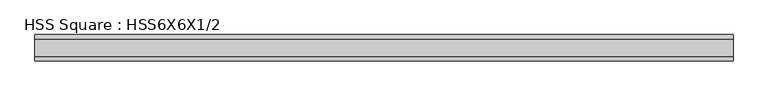
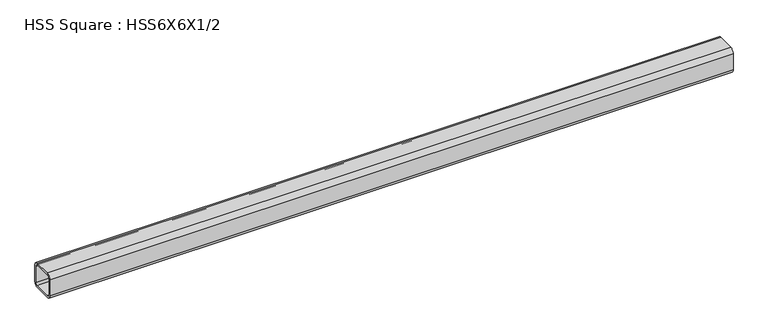
"""IFC4 building model written with IfcOpenShell, lengths in millimetres: member geometry, HSS Square : HSS6X6X1/2."""

from ifc_helpers import new_model, si_unit, point, frame, frame_2d, origin, place, context, project, spatial, polyline, circle_curve, trimmed, segment, composite_curve, outline, extrude, source, transform, mapped, element, save


def hss_square_hss6x6x1_2_d64262a5(model_context):
    return source(origin(), model_context, "Body", "SweptSolid", [
        extrude(outline(composite_curve([segment(polyline([(76.2, 50.8), (76.2, -50.8)]), True, "CONTINUOUS"), segment(trimmed(circle_curve(frame_2d((50.8, -50.8)), 25.4), [point((76.2, -50.8))], [point((50.8, -76.2))], False, "CARTESIAN"), True, "CONTINUOUS"), segment(polyline([(50.8, -76.2), (-50.8, -76.2)]), True, "CONTINUOUS"), segment(trimmed(circle_curve(frame_2d((-50.8, -50.8)), 25.4), [point((-50.8, -76.2))], [point((-76.2, -50.8))], False, "CARTESIAN"), True, "CONTINUOUS"), segment(polyline([(-76.2, -50.8), (-76.2, 50.8)]), True, "CONTINUOUS"), segment(trimmed(circle_curve(frame_2d((-50.8, 50.8)), 25.4), [point((-76.2, 50.8))], [point((-50.8, 76.2))], False, "CARTESIAN"), True, "CONTINUOUS"), segment(polyline([(-50.8, 76.2), (50.8, 76.2)]), True, "CONTINUOUS"), segment(trimmed(circle_curve(frame_2d((50.8, 50.8)), 25.4), [point((50.8, 76.2))], [point((76.2, 50.8))], False, "CARTESIAN"), True, "CONTINUOUS")], self_intersect=False), holes=[composite_curve([segment(trimmed(circle_curve(frame_2d((-50.8, 50.8)), 12.7), [point((-50.8, 63.5))], [point((-63.5, 50.8))], True, "CARTESIAN"), True, "CONTINUOUS"), segment(polyline([(-63.5, 50.8), (-63.5, -50.8)]), True, "CONTINUOUS"), segment(trimmed(circle_curve(frame_2d((-50.8, -50.8)), 12.7), [point((-63.5, -50.8))], [point((-50.8, -63.5))], True, "CARTESIAN"), True, "CONTINUOUS"), segment(polyline([(-50.8, -63.5), (50.8, -63.5)]), True, "CONTINUOUS"), segment(trimmed(circle_curve(frame_2d((50.8, -50.8)), 12.7), [point((50.8, -63.5))], [point((63.5, -50.8))], True, "CARTESIAN"), True, "CONTINUOUS"), segment(polyline([(63.5, -50.8), (63.5, 50.8)]), True, "CONTINUOUS"), segment(trimmed(circle_curve(frame_2d((50.8, 50.8)), 12.7), [point((63.5, 50.8))], [point((50.8, 63.5))], True, "CARTESIAN"), True, "CONTINUOUS"), segment(polyline([(50.8, 63.5), (-50.8, 63.5)]), True, "CONTINUOUS")], self_intersect=False)]), frame((-2084.0805216, 0.0, 0.0), z_axis=(1.0, 0.0, 0.0), x_axis=(0.0, 1.0, 0.0)), (0.0, 0.0, 1.0), 4048.5285365),
    ])


if __name__ == "__main__":
    model = new_model("IFC4")
    model_context = context("Model", 3, world=origin())
    ifc_project = project(units=[si_unit("LENGTHUNIT", "METRE", prefix="MILLI")], contexts=[model_context])
    site = spatial("IfcSite", under=ifc_project)
    building = spatial("IfcBuilding", under=site)
    placement = place(None, origin())
    hss_square_hss6x6x1_2_shape = hss_square_hss6x6x1_2_d64262a5(model_context)
    element("IfcMember", 1, ObjectType="HSS Square : HSS6X6X1/2", at=placement, inside=building, context=model_context, shape_type="MappedRepresentation", body=[
        mapped(hss_square_hss6x6x1_2_shape, transform((0.0, 0.0, 0.0), x_axis=(1.0, 0.0, 0.0), y_axis=(0.0, 1.0, 0.0), z_axis=(0.0, 0.0, 1.0))),
    ])
    save(model, "model.ifc")

# Revit data of these elements
# Type "HSS Square : HSS6X6X1/2"
#   Section Name Key = "HSS 6X6X1/2"
#   Assembly Code = "B10"
#   Width = 6.000"
#   Wall Nominal Thickness = 0.500"
#   Wall Design Thickness = 0.465"
#   Torsional Moment of Inertia = 81.10 in⁴
#   Torsional Modulus = 28.10 in³
#   Section Area = 9.74 in²
#   Plastic Modulus weak axis = 19.80 in³
#   Plastic Modulus strong axis = 19.80 in³
#   Outer Fillet = 1.000"
#   Nominal Weight = 35.24 lbf/ft
#   Moment of Inertia weak axis = 48.30 in⁴
#   Moment of Inertia strong axis = 48.30 in⁴
#   Inner Fillet = 0.500"
#   Height = 6.000"
#   Elastic Modulus weak axis = 16.10 in³
#   Elastic Modulus strong axis = 16.10 in³
#   Centroid Vertical = 3.000"
#   Centroid Horizontal = 3.000"
#   Length [instance default] = 5' - 0"
#   Structural Material [instance default] = Steel ASTM A500, Grade B, Rectangular and Square
#   Principal Axes Angle = 0
# Element 1 (IfcMember, "HSS Square : HSS6X6X1/2")
#   Structural Material = Steel ASTM A992
#   Materials on its faces: "Steel ASTM A992"
# Materials
#   "Steel ASTM A500, Grade B, Rectangular and Square": class "Metal", colour RGB 199 199 199, transparency 0, Description = "Carbon steel", Cost = 0
#   "Steel ASTM A992": class "Metal", colour RGB 199 199 199, transparency 0, Description = "Structural steel 50ksi", Cost = 0
